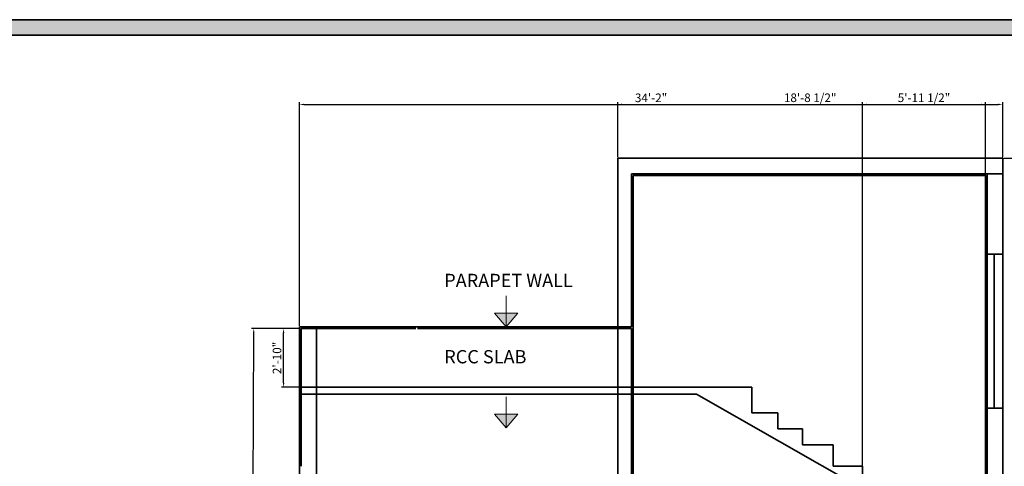
# Model space of a CAD drawing. Units: inches. Extents: x 1804 to 3296, y 909 to 2477.
# Tile 30 of 31: x 2434 to 3008, y 2216 to 2477. Entities that reach past the tile are written whole.
import ezdxf

# ---------------------------------------------------------------- set-up
doc = ezdxf.new("R2010")
doc.units = ezdxf.units.IN
for name, color, linetype, lineweight in [('A-ANNO-DIMS', 2, 'Continuous', 18), ('A-ANNO-SYMB', 7, 'Continuous', 18), ('A-ANNO-TTLB', 156, 'Continuous', 35), ('A-WALL-PATT', 10, 'Continuous', 13), ('SEC', 160, 'Continuous', 35), ('TEXT', 190, 'Continuous', 18)]:
    doc.layers.add(name, color=color, linetype=linetype, lineweight=lineweight)
doc.styles.get("Standard").update_dxf_attribs({"font": 'arial.ttf'})
doc.dimstyles.new('ISO-25', dxfattribs={"dimtxt": 5, "dimasz": 2.5, "dimexe": 1.25, "dimexo": 0.625, "dimtad": 1, "dimdec": 0, "dimlunit": 4, "dimtxsty": 'Standard', "dimcen": 2.5, "dimadec": 0, "dimazin": 0, "dimtfac": 1, "dimtdec": 0, "dimtmove": 0, "dimatfit": 3, "dimfxl": 1, "dimarcsym": 0})

# ---------------------------------------------------------------- blocks, each defined once
blk = doc.blocks.new('*D33')
at = {"layer": 'A-ANNO-DIMS', "color": 0, "lineweight": -2, "transparency": 16777216}
for p, q in [((3007.45, 2395.8), (3058.21, 2395.8)), ((3056.96, 1983.77), (3056.96, 2393.3)), ((3007.45, 1981.27), (3058.21, 1981.27))]:
    blk.add_line(p, q, dxfattribs=at)
at = {"layer": 'A-ANNO-DIMS', "color": 0, "lineweight": 100, "transparency": 16777216}
for points in [[(3056.55, 2393.3), (3057.38, 2393.3), (3056.96, 2395.8)], [(3056.55, 1983.77), (3057.38, 1983.77), (3056.96, 1981.27)]]:
    blk.add_solid(points, dxfattribs=at)
at = {"layer": 'Defpoints', "color": 0, "lineweight": 100, "transparency": 16777216}
for p in [(3006.82, 2395.8), (3056.96, 2395.8), (3006.82, 1981.27)]:
    blk.add_point(p, dxfattribs=at)
at = {"layer": 'A-ANNO-DIMS', "color": 0, "transparency": 16777216, "insert": (3053.79, 2188.53), "char_height": 5, "attachment_point": 5, "rotation": 90}
blk.add_mtext('34\'-7"', dxfattribs=at)
blk = doc.blocks.new('*D34')
at = {"layer": 'A-ANNO-DIMS', "color": 0, "lineweight": -2, "transparency": 16777216}
for p, q in [((2597.24, 2296.57), (2568.96, 2296.69)), ((2569.22, 2055.41), (2570.2, 2294.18)), ((2596.24, 2052.8), (2567.96, 2052.92))]:
    blk.add_line(p, q, dxfattribs=at)
at = {"layer": 'A-ANNO-DIMS', "color": 0, "lineweight": 100, "transparency": 16777216}
for points in [[(2569.78, 2294.19), (2570.61, 2294.18), (2570.21, 2296.68)], [(2568.8, 2055.41), (2569.64, 2055.41), (2569.21, 2052.91)]]:
    blk.add_solid(points, dxfattribs=at)
at = {"layer": 'Defpoints', "color": 0, "lineweight": 100, "transparency": 16777216}
for p in [(2570.21, 2296.68), (2597.87, 2296.57), (2596.87, 2052.8)]:
    blk.add_point(p, dxfattribs=at)
at = {"layer": 'A-ANNO-DIMS', "color": 0, "transparency": 16777216, "insert": (2566.53, 2174.81), "char_height": 5, "attachment_point": 5, "rotation": 89.76496}
blk.add_mtext('20\'-4"', dxfattribs=at)
blk = doc.blocks.new('*D35')
at = {"layer": 'A-ANNO-DIMS', "color": 0, "lineweight": -2, "transparency": 16777216}
for p, q in [((2597.24, 2296.57), (2586.36, 2296.57)), ((2587.61, 2264.89), (2587.61, 2294.07)), ((2597.24, 2262.39), (2586.36, 2262.39))]:
    blk.add_line(p, q, dxfattribs=at)
at = {"layer": 'A-ANNO-DIMS', "color": 0, "lineweight": 100, "transparency": 16777216}
for points in [[(2587.19, 2294.07), (2588.03, 2294.07), (2587.61, 2296.57)], [(2587.19, 2264.89), (2588.03, 2264.89), (2587.61, 2262.39)]]:
    blk.add_solid(points, dxfattribs=at)
at = {"layer": 'Defpoints', "color": 0, "lineweight": 100, "transparency": 16777216}
for p in [(2587.61, 2296.57), (2597.87, 2296.57), (2597.87, 2262.39)]:
    blk.add_point(p, dxfattribs=at)
at = {"layer": 'A-ANNO-DIMS', "color": 0, "transparency": 16777216, "insert": (2584.43, 2279.48), "char_height": 5, "attachment_point": 5, "rotation": 90}
blk.add_mtext('2\'-10"', dxfattribs=at)
blk = doc.blocks.new('SECTION-NOTE-ARROW')
h = blk.add_hatch(color=256)
h.dxf.hatch_style = 1
h.paths.add_polyline_path([(6.75, 8.05), (0, 8.05), (6.75, 0)])
h.paths.add_polyline_path([(13.51, 8.05), (6.75, 8.05), (6.75, 0)])
for p, q in [((6.75, 18.17), (6.75, 0)), ((6.75, 0), (0, 8.05)), ((0, 8.05), (13.51, 8.05)), ((6.75, 0), (13.51, 8.05))]:
    blk.add_line(p, q)
blk = doc.blocks.new('*D88')
at = {"layer": 'A-ANNO-DIMS', "color": 0, "lineweight": -2, "transparency": 16777216}
for p, q in [((2596.87, 2298.2), (2596.87, 2428.45)), ((3006.82, 2396.42), (3006.82, 2428.45)), ((2599.37, 2427.2), (3004.32, 2427.2))]:
    blk.add_line(p, q, dxfattribs=at)
at = {"layer": 'A-ANNO-DIMS', "color": 0, "lineweight": 100, "transparency": 16777216}
for points in [[(2599.37, 2427.61), (2599.37, 2426.78), (2596.87, 2427.2)], [(3004.32, 2427.61), (3004.32, 2426.78), (3006.82, 2427.2)]]:
    blk.add_solid(points, dxfattribs=at)
at = {"layer": 'Defpoints', "color": 0, "lineweight": 100, "transparency": 16777216}
for p in [(3006.82, 2427.2), (3006.82, 2395.8), (2596.87, 2297.57)]:
    blk.add_point(p, dxfattribs=at)
at = {"layer": 'A-ANNO-DIMS', "color": 0, "transparency": 16777216, "insert": (2801.84, 2430.38), "char_height": 5, "attachment_point": 5}
blk.add_mtext('34\'-2"', dxfattribs=at)
blk = doc.blocks.new('*D89')
at = {"layer": 'A-ANNO-DIMS', "color": 0, "lineweight": -2, "transparency": 16777216}
for p, q in [((2782.37, 2396.42), (2782.37, 2428.45)), ((3006.82, 2396.42), (3006.82, 2428.45)), ((2784.87, 2427.2), (3004.32, 2427.2))]:
    blk.add_line(p, q, dxfattribs=at)
at = {"layer": 'A-ANNO-DIMS', "color": 0, "lineweight": 100, "transparency": 16777216}
for points in [[(2784.87, 2427.61), (2784.87, 2426.78), (2782.37, 2427.2)], [(3004.32, 2427.61), (3004.32, 2426.78), (3006.82, 2427.2)]]:
    blk.add_solid(points, dxfattribs=at)
at = {"layer": 'Defpoints', "color": 0, "lineweight": 100, "transparency": 16777216}
for p in [(3006.82, 2427.2), (2782.37, 2395.8), (3006.82, 2395.8)]:
    blk.add_point(p, dxfattribs=at)
at = {"layer": 'A-ANNO-DIMS', "color": 0, "transparency": 16777216, "insert": (2894.59, 2430.41), "char_height": 5, "attachment_point": 5}
blk.add_mtext('18\'-8 1/2"', dxfattribs=at)
blk = doc.blocks.new('*D92')
at = {"layer": 'A-ANNO-DIMS', "color": 0, "lineweight": -2, "transparency": 16777216}
for p, q in [((2925.08, 2203.82), (2925.08, 2428.45)), ((2996.82, 2203.82), (2996.82, 2428.45)), ((2927.58, 2427.2), (2994.32, 2427.2))]:
    blk.add_line(p, q, dxfattribs=at)
at = {"layer": 'A-ANNO-DIMS', "color": 0, "lineweight": 100, "transparency": 16777216}
for points in [[(2927.58, 2427.61), (2927.58, 2426.78), (2925.08, 2427.2)], [(2994.32, 2427.61), (2994.32, 2426.78), (2996.82, 2427.2)]]:
    blk.add_solid(points, dxfattribs=at)
at = {"layer": 'Defpoints', "color": 0, "lineweight": 100, "transparency": 16777216}
for p in [(2996.82, 2427.2), (2925.08, 2203.2), (2996.82, 2203.2)]:
    blk.add_point(p, dxfattribs=at)
at = {"layer": 'A-ANNO-DIMS', "color": 0, "transparency": 16777216, "insert": (2960.95, 2430.41), "char_height": 5, "attachment_point": 5}
blk.add_mtext('5\'-11 1/2"', dxfattribs=at)

msp = doc.modelspace()

# ---------------------------------------------------------------- hatches: boundary and pattern name
at = {"layer": 'A-ANNO-TTLB'}
h = msp.add_hatch(color=256, dxfattribs=at)
h.dxf.hatch_style = 1
h.paths.add_polyline_path([(3294.53, 2476.54), (1803.79, 2476.54), (1805.43, 909.47), (3296.17, 909.47)])
h.paths.add_polyline_path([(1811, 914.33), (1812.79, 2467.54), (3285.53, 2467.54), (3283.74, 914.33)], flags=16)
h.paths.add_polyline_path([(1925.58, 1062.77), (1925.58, 1138.07), (1925.58, 1539.88), (1925.58, 1793.38), (1925.58, 1830.04), (2325.54, 1830.04), (2325.54, 1793.38), (2325.54, 1586.42), (2325.54, 1138.07), (2325.54, 1062.77)], flags=0)
h.paths.add_polyline_path([(1997.22, 1029.4), (2008.85, 1037.96), (2008.85, 1020.84)], flags=0)
h.paths.add_polyline_path([(1934.58, 1138.07), (1934.58, 1147.07), (2078.77, 1147.07), (2078.77, 1138.07), (2060.94, 1138.07)], flags=0)
h.paths.add_polyline_path([(1944.35, 1138.07), (1944.35, 1147.07), (2056.05, 1147.07), (2056.05, 1138.07)], flags=0)
h.paths.add_polyline_path([(2222.24, 1037.96), (2233.87, 1029.4), (2222.24, 1020.84)], flags=0)
h.paths.add_polyline_path([(2061.94, 1139.07), (2061.94, 1146.07), (2077.77, 1146.07), (2077.77, 1139.07)], flags=0)
h.paths.add_polyline_path([(2149.58, 1138.07), (2149.58, 1269.44), (2158.58, 1269.44), (2158.58, 1326.69), (2149.58, 1326.69), (2149.58, 1340.94), (2139.6, 1340.94), (2139.6, 1434.25), (2149.58, 1434.25), (2149.58, 1447.36), (2158.58, 1447.36), (2158.58, 1423.87), (2158.58, 1408.06), (2198.46, 1408.06), (2198.46, 1412.56), (2282.65, 1412.56), (2282.65, 1465.94), (2316.54, 1465.94), (2316.54, 1590.92), (2192.86, 1590.92), (2192.86, 1595.3), (2291.17, 1595.3), (2291.17, 1590.92), (2316.54, 1590.92), (2316.54, 1784.38), (2300.24, 1784.38), (2300.24, 1757.47), (2268, 1757.47), (2268, 1681.04), (2180.87, 1681.04), (2180.87, 1757.47), (2148.63, 1757.47), (2148.63, 1784.38), (2119.08, 1784.38), (2119.08, 1585.58), (2114.58, 1585.58), (2114.58, 1784.38), (2064.11, 1784.38), (2046.28, 1784.38), (2046.28, 1760.38), (1958.58, 1760.38), (1958.58, 1664.38), (1934.58, 1664.38), (1934.58, 1784.38), (1934.58, 1793.38), (2046.28, 1793.38), (2064.11, 1793.38), (2119.08, 1793.38), (2230.78, 1793.38), (2230.78, 1784.38), (2268, 1784.38), (2300.24, 1784.38), (2316.54, 1784.38), (2316.54, 1590.92), (2316.54, 1373.73), (2316.54, 1138.07)], flags=0)
h.paths.add_polyline_path([(2209.19, 1166.63), (2209.19, 1175.63), (2158.58, 1175.63), (2209.19, 1223.63), (2209.19, 1231.63), (2183.88, 1231.63), (2183.88, 1301.66), (2242.59, 1301.66), (2242.59, 1326.69), (2316.54, 1326.69), (2272.59, 1271.63), (2272.59, 1223.63), (2316.54, 1175.63), (2272.59, 1175.63), (2272.59, 1166.63)], flags=0)
h.paths.add_polyline_path([(1947.77, 1345.22), (1947.77, 1457.48), (1991.2, 1457.48), (1991.2, 1451.7), (1991.2, 1352.18), (1991.2, 1345.22)], flags=0)
h.paths.add_polyline_path([(2209.19, 1271.63), (2262.59, 1271.63), (2262.59, 1311.85), (2272.59, 1301.66), (2272.59, 1271.63), (2269.92, 1269.63), (2270.59, 1269.63), (2270.59, 1225.63), (2211.19, 1225.63), (2211.19, 1269.63), (2211.86, 1269.63)], flags=0)
h.paths.add_polyline_path([(2000.34, 1378.21), (2000.34, 1429.71), (2025.22, 1429.71), (2025.22, 1378.21)], flags=0)
h.paths.add_polyline_path([(2001.34, 1379.21), (2001.34, 1428.71), (2024.22, 1428.71), (2024.22, 1379.21)], flags=0)
h.paths.add_polyline_path([(2012.34, 1390.21), (2012.34, 1417.71), (2013.22, 1417.71), (2013.22, 1390.21)], flags=0)
h.paths.add_polyline_path([(2237.56, 1331.19), (2237.56, 1340.18), (2238.62, 1340.18), (2238.62, 1386.84), (2241.04, 1386.84), (2242.06, 1386.84), (2242.06, 1408.06), (2316.54, 1331.19)], flags=0)
h.paths.add_polyline_path([(1953.73, 1464.35), (1953.73, 1498.59), (1981.74, 1498.59), (1981.74, 1464.35)], flags=0)
h.paths.add_polyline_path([(1987.63, 1462.08), (1987.63, 1500.95), (2104.07, 1500.95), (2104.07, 1462.08), (2099.27, 1462.08), (1993.6, 1462.08)], flags=0)
h.paths.add_polyline_path([(1956.06, 1481.47, -1), (1979.41, 1481.47, -1)], flags=0)
edge = h.paths.add_edge_path(flags=0)
edge.add_ellipse((2299.53, 1438.37), major_axis=(0.31, 21.36), ratio=0.670333, start_angle=0, end_angle=360)
h.paths.add_polyline_path([(2297.39, 1438.37, -1), (2301.67, 1438.37, -1)], flags=0)
h.paths.add_polyline_path([(2591.54, 1163.23), (2591.54, 1179.38), (2591.54, 1379.68), (2591.54, 1395.84), (2734.5, 1395.84), (2734.5, 1379.68), (2734.5, 1179.38), (2734.5, 1163.23)], flags=0)
h.paths.add_polyline_path([(2592.54, 1164.23), (2592.54, 1166.23), (2733.5, 1166.23), (2733.5, 1164.23)], flags=0)
h.paths.add_polyline_path([(2592.54, 1180.38), (2592.54, 1378.68), (2733.5, 1378.68), (2733.5, 1180.38)], flags=0)
h.paths.add_polyline_path([(2593.54, 1181.38), (2593.54, 1377.68), (2732.5, 1377.68), (2732.5, 1181.38)], flags=0)
h.paths.add_polyline_path([(2594.54, 1182.38), (2594.54, 1376.68), (2731.5, 1376.68), (2731.5, 1182.38)], flags=0)
h.paths.add_polyline_path([(1936.95, 1697.46), (1936.95, 1736.46), (1955.41, 1736.46), (1955.41, 1697.46)], flags=0)
h.paths.add_polyline_path([(1938.48, 1718.36), (1938.48, 1734.92), (1953.65, 1734.92), (1953.65, 1718.36)], flags=0)
h.paths.add_polyline_path([(1944.75, 1726.64, -1), (1947.37, 1726.64, -1)], flags=0)
h.paths.add_polyline_path([(2592.54, 1394.84), (2733.5, 1394.84), (2733.5, 1392.84), (2592.54, 1392.84)], flags=0)
h.paths.add_polyline_path([(1976.61, 1762.5), (1976.61, 1781.44), (2012.79, 1781.44), (2012.79, 1762.5)], flags=0)
h.paths.add_polyline_path([(1979.57, 1771.97, -1), (1991.39, 1771.97, -1)], flags=0)
h.paths.add_polyline_path([(1995.36, 1771.97, -1), (2007.18, 1771.97, -1)], flags=0)
h.paths.add_polyline_path([(2251.51, 1744.53), (2268, 1730.05), (2251.51, 1730.05)], flags=0)
h.paths.add_polyline_path([(2047.28, 1785.38), (2047.28, 1792.38), (2063.11, 1792.38), (2063.11, 1785.38)], flags=0)
h.paths.add_polyline_path([(2155.08, 1770.92, -1), (2174.42, 1770.92, -1)], flags=0)
h.paths.add_polyline_path([(2188.59, 1758.27), (2188.59, 1772.81), (2222.3, 1772.81), (2222.3, 1758.27)], flags=0)
h.paths.add_polyline_path([(2223.97, 1758.27), (2223.97, 1772.81), (2257.68, 1772.81), (2257.68, 1758.27)], flags=0)
h.paths.add_polyline_path([(2274.45, 1770.92, -1), (2293.8, 1770.92, -1)], flags=0)
h.paths.add_polyline_path([(2591.54, 1582.09), (2591.54, 1782.39), (2734.5, 1782.39), (2734.5, 1582.09)], flags=0)
h.paths.add_polyline_path([(2592.54, 1583.09), (2592.54, 1781.39), (2733.5, 1781.39), (2733.5, 1583.09)], flags=0)
h.paths.add_polyline_path([(2593.54, 1584.09), (2593.54, 1780.39), (2732.5, 1780.39), (2732.5, 1584.09)], flags=0)
h.paths.add_polyline_path([(2594.54, 1585.09), (2594.54, 1779.39), (2731.5, 1779.39), (2731.5, 1585.09)], flags=0)
h.paths.add_polyline_path([(1922.17, 1978.79), (1922.17, 2295.08), (1922.17, 2296.08), (2115.67, 2296.08), (2115.67, 2384.31), (2115.67, 2385.31), (2322.12, 2385.31), (2323.12, 2385.31), (2323.12, 1979.79), (2323.12, 1978.79), (1923.17, 1978.79)], flags=0)
h.paths.add_polyline_path([(1922.17, 1978.79), (1922.17, 2051.31), (1922.17, 2214.86), (1922.17, 2296.08), (2115.67, 2296.08), (2115.67, 2385.31), (2323.12, 2385.31), (2323.12, 2280.42), (2323.12, 1978.79), (2115.67, 1978.79)], flags=0)
h.paths.add_polyline_path([(1923.17, 1979.79), (1923.17, 2050.31), (2115.67, 2050.31), (2115.67, 2051.31), (1923.17, 2051.31), (1923.17, 2213.86), (1923.17, 2214.86), (1923.17, 2295.08), (1990.02, 2295.08), (1990.02, 2214.86), (1991.02, 2214.86), (1991.02, 2295.08), (2115.67, 2295.08), (2115.67, 1979.79), (2116.67, 1979.79), (2116.67, 2304.18), (2116.67, 2384.31), (2322.12, 2384.31), (2322.12, 2280.42), (2322.12, 1979.79), (2115.67, 1979.79)], flags=0)
h.paths.add_polyline_path([(2972.46, 1192.5), (2972.46, 1196.92), (2995.47, 1196.92), (2995.47, 1255.47), (2995.09, 1255.47), (2987.42, 1249.39), (2980.08, 1255.47), (2978.05, 1255.47), (2978.05, 1257.24), (2995.47, 1257.24), (2995.47, 1261.58), (3015.37, 1261.58), (3015.37, 1333.28), (3015.37, 1414.4), (3032.82, 1414.4), (3032.82, 1333.28), (3032.82, 1261.58), (3052.66, 1261.58), (3052.66, 1255.47), (3079.86, 1255.47), (3078.72, 1254.57), (3081.47, 1252.29), (3078.56, 1249.99), (3075.81, 1252.26), (3072.57, 1249.69), (3070.36, 1251.52), (3067.67, 1249.39), (3060.34, 1255.47), (3052.66, 1255.47), (3052.66, 1196.92), (3054.58, 1196.92), (3074, 1196.92), (3074, 1192.5), (3052.66, 1192.5), (2995.47, 1192.5)], flags=0)
h.paths.add_polyline_path([(2490.75, 1979.27), (2490.75, 1980.27), (2596.87, 1980.27), (2596.87, 2051.8), (2596.87, 2052.8), (2596.87, 2216.35), (2596.87, 2297.57), (2717.32, 2297.57), (2710.57, 2305.62), (2724.07, 2305.62), (2717.32, 2297.57), (2782.37, 2297.57), (2782.37, 2395.8), (3006.82, 2395.8), (3006.82, 1981.27), (3093.73, 1981.27), (3093.73, 1980.27), (3047.51, 1980.27), (3046.37, 1979.37), (3049.11, 1977.1), (3046.2, 1974.79), (3043.46, 1977.07), (3040.21, 1974.49), (3038, 1976.32), (3035.32, 1974.2), (3027.98, 1980.27), (2871.83, 1980.27), (2871.83, 1981.27), (2791.37, 1981.27), (2791.37, 2050.8), (2597.87, 2050.8), (2597.87, 1980.27), (2597.87, 1979.27), (2546.27, 1979.27), (2545.12, 1978.37), (2547.87, 1976.1), (2544.96, 1973.79), (2542.22, 1976.07), (2538.97, 1973.49), (2536.76, 1975.32), (2534.07, 1973.2), (2526.74, 1979.27)], flags=0)
h.paths.add_polyline_path([(2597.87, 2051.8), (2606.87, 2051.8), (2606.87, 2258.39), (2597.87, 2258.39), (2597.87, 2296.57), (2606.87, 2296.57), (2606.87, 2262.39), (2782.37, 2262.39), (2782.37, 2296.57), (2790.37, 2296.57), (2790.37, 2262.39), (2791.37, 2262.39), (2791.37, 2305.67), (2791.37, 2385.8), (2996.82, 2385.8), (2996.82, 2339.85), (3006.82, 2339.85), (3006.82, 2250.12), (2997.82, 2250.12), (2997.82, 1981.27), (2996.82, 1981.27), (2872.83, 1981.27), (2872.83, 1991.8), (2871.83, 1991.8), (2871.83, 2050.8), (2790.37, 2050.8), (2597.87, 2050.8)], flags=0)
h.paths.add_polyline_path([(2179.93, 2153.92), (2179.93, 2353.97), (2259.98, 2353.97), (2259.98, 2153.92)], flags=0)
h.paths.add_polyline_path([(2180.93, 2154.92), (2180.93, 2352.97), (2258.98, 2352.97), (2258.98, 2154.92)], flags=0)
h.paths.add_polyline_path([(2960.87, 1608.49), (2960.87, 1753.62), (3070.9, 1753.62), (3070.9, 1608.49)], flags=0)
h.paths.add_polyline_path([(2961.87, 1609.49), (2961.87, 1752.62), (3069.9, 1752.62), (3069.9, 1609.49)], flags=0)
h.paths.add_polyline_path([(2962.87, 1610.49), (2962.87, 1751.62), (3068.9, 1751.62), (3068.9, 1610.49)], flags=0)
h.paths.add_polyline_path([(2963.87, 1611.49), (2963.87, 1750.62), (3067.9, 1750.62), (3067.9, 1611.49)], flags=0)
h.paths.add_polyline_path([(2782.37, 2051.8), (2782.37, 2216.32), (2791.37, 2216.32), (2791.37, 2051.8), (2872.83, 2051.8), (2872.83, 2068.56), (2884.67, 2068.56), (2884.67, 2085.33), (2896.51, 2085.33), (2896.51, 2102.09), (2908.36, 2102.09), (2908.36, 2118.85), (2920.2, 2118.85), (2920.2, 2135.62), (2932.05, 2135.62), (2932.05, 2145.3), (2925.08, 2145.3), (2925.08, 2203.2), (2996.82, 2203.2), (2996.82, 2145.3), (2953.82, 2145.3), (2872.83, 2051.8), (2790.37, 2051.8)], flags=0)
h.paths.add_polyline_path([(2717.32, 2238.65), (2710.57, 2246.7), (2724.07, 2246.7)], flags=0)
h.paths.add_polyline_path([(2003.09, 1122.79), (2017.16, 1122.79), (2017.16, 1138.74), (2003.09, 1138.74)], flags=8)
h.paths.add_polyline_path([(2174.76, 1792.72), (2188.83, 1792.72), (2188.83, 1808.66), (2174.76, 1808.66)], flags=8)
h.paths.add_polyline_path([(1987.95, 1792.51), (2002.02, 1792.51), (2002.02, 1808.45), (1987.95, 1808.45)], flags=8)
h.paths.add_polyline_path([(2148.79, 1289.26), (2160.46, 1289.26), (2160.46, 1305.2), (2148.79, 1305.2)], flags=8)
h.paths.add_polyline_path([(2115.36, 1133.57), (2127.04, 1133.57), (2127.04, 1149.51), (2115.36, 1149.51)], flags=8)
h.paths.add_polyline_path([(2237.58, 1421.48), (2249.25, 1421.48), (2249.25, 1437.43), (2237.58, 1437.43)], flags=8)
h.paths.add_polyline_path([(2134.99, 1584.32), (2146.66, 1584.32), (2146.66, 1600.26), (2134.99, 1600.26)], flags=8)
h.paths.add_polyline_path([(2101.95, 1557.31), (2113.62, 1557.31), (2113.62, 1573.25), (2101.95, 1573.25)], flags=8)
h.paths.add_polyline_path([(2937.85, 1156.77), (3120.41, 1156.77), (3120.41, 1185.72), (2937.85, 1185.72)], flags=8)
h.paths.add_polyline_path([(2980.71, 1786.71), (3050.06, 1786.71), (3050.06, 1802.66), (2980.71, 1802.66)], flags=8)
h.paths.add_polyline_path([(2869.28, 1661.96), (2938.62, 1661.96), (2938.62, 1690.8), (2869.28, 1690.8)], flags=8)
h.paths.add_polyline_path([(3092.27, 1674.86), (3161.62, 1674.86), (3161.62, 1690.8), (3092.27, 1690.8)], flags=8)
h.paths.add_polyline_path([(2980.71, 1674.86), (3050.06, 1674.86), (3050.06, 1690.8), (2980.71, 1690.8)], flags=8)
h.paths.add_polyline_path([(2649.07, 1678.23), (2674.53, 1678.23), (2674.53, 1714.76), (2649.07, 1714.76)], flags=8)
h.paths.add_polyline_path([(2530.84, 1981.63), (2549.13, 1981.63), (2549.13, 1997.57), (2530.84, 1997.57)], flags=8)
h.paths.add_polyline_path([(3031.29, 1981.77), (3049.58, 1981.77), (3049.58, 1997.71), (3031.29, 1997.71)], flags=8)
h.paths.add_polyline_path([(2715.38, 1911.9), (2851.54, 1911.9), (2851.54, 1940.85), (2715.38, 1940.85)], flags=8)
h.paths.add_polyline_path([(2015.23, 1927.36), (2205.42, 1927.36), (2205.42, 1956.3), (2015.23, 1956.3)], flags=8)
h.paths.add_polyline_path([(2671.84, 2057.84), (2702.75, 2057.84), (2702.75, 2073.79), (2671.84, 2073.79)], flags=8)
h.paths.add_polyline_path([(2678.5, 2316.52), (2765.26, 2316.52), (2765.26, 2332.46), (2678.5, 2332.46)], flags=8)
h.paths.add_polyline_path([(2678.48, 2271.96), (2736.41, 2271.96), (2736.41, 2287.9), (2678.48, 2287.9)], flags=8)
h.paths.add_polyline_path([(2019.2, 972.79), (2243.21, 972.79), (2243.21, 1001.74), (2019.2, 1001.74)], flags=8)
h.paths.add_polyline_path([(2097.06, 1021.56), (2132.16, 1021.56), (2132.16, 1037.51), (2097.06, 1037.51)], flags=8)
h.paths.add_polyline_path([(2182.47, 1360.48), (2207.35, 1360.48), (2207.35, 1376.42), (2182.47, 1376.42)], flags=8)
h.paths.add_polyline_path([(2261.12, 1361.77), (2295.01, 1361.77), (2295.01, 1377.71), (2261.12, 1377.71)], flags=8)
h.paths.add_polyline_path([(2245.75, 1511.51), (2278.44, 1511.51), (2278.44, 1527.46), (2245.75, 1527.46)], flags=8)
h.paths.add_polyline_path([(1991.16, 1296.29), (2060.51, 1296.29), (2060.51, 1312.23), (1991.16, 1312.23)], flags=8)
h.paths.add_polyline_path([(2187, 1651.35), (2246.71, 1651.35), (2246.71, 1667.29), (2187, 1667.29)], flags=8)
h.paths.add_polyline_path([(1976.49, 1684.81), (2068.63, 1684.81), (2068.63, 1700.76), (1976.49, 1700.76)], flags=8)
at = {"layer": 'A-WALL-PATT'}
h = msp.add_hatch(color=256, dxfattribs=at)
h.dxf.hatch_style = 1
h.paths.add_polyline_path([(2119.08, 1544.38), (1925.58, 1544.38), (1925.58, 1539.88), (2119.08, 1539.88)])
h.paths.add_polyline_path([(2119.08, 1545.58), (2114.58, 1545.58), (2114.58, 1544.38), (2119.08, 1544.38)])
h.paths.add_polyline_path([(1965.87, 1658.79), (1965.87, 1679.09), (1955.57, 1679.09), (1955.57, 1658.79)], flags=9)
h.paths.add_polyline_path([(2293.18, 1677.29), (2293.18, 1697.58), (2282.88, 1697.58), (2282.88, 1677.29)], flags=9)
h.paths.add_polyline_path([(2271.13, 1545.23), (2287.53, 1545.23), (2287.53, 1555.53), (2271.13, 1555.53)], flags=9)
h.paths.add_polyline_path([(2303.26, 1488.52), (2303.26, 1508.82), (2292.95, 1508.82), (2292.95, 1488.52)], flags=9)
h.paths.add_polyline_path([(2271.13, 1393.15), (2287.53, 1393.15), (2287.53, 1403.45), (2271.13, 1403.45)], flags=9)
h.paths.add_polyline_path([(2306.48, 1361.45), (2306.48, 1377.86), (2296.18, 1377.86), (2296.18, 1361.45)], flags=9)
h.paths.add_polyline_path([(2174.54, 1361.45), (2174.54, 1377.86), (2164.23, 1377.86), (2164.23, 1361.45)], flags=9)
h.paths.add_polyline_path([(1968.21, 1333.34), (1968.21, 1353.64), (1957.91, 1353.64), (1957.91, 1333.34)], flags=9)
h.paths.add_polyline_path([(2003.09, 1122.79), (2017.16, 1122.79), (2017.16, 1138.74), (2003.09, 1138.74)], flags=9)
h.paths.add_polyline_path([(2174.76, 1792.72), (2188.83, 1792.72), (2188.83, 1808.66), (2174.76, 1808.66)], flags=9)
h.paths.add_polyline_path([(1987.95, 1792.51), (2002.02, 1792.51), (2002.02, 1808.45), (1987.95, 1808.45)], flags=9)
h.paths.add_polyline_path([(2148.79, 1289.26), (2160.46, 1289.26), (2160.46, 1305.2), (2148.79, 1305.2)], flags=9)
h.paths.add_polyline_path([(2115.36, 1133.57), (2127.04, 1133.57), (2127.04, 1149.51), (2115.36, 1149.51)], flags=9)
h.paths.add_polyline_path([(2237.58, 1421.48), (2249.25, 1421.48), (2249.25, 1437.43), (2237.58, 1437.43)], flags=9)
h.paths.add_polyline_path([(2134.99, 1584.32), (2146.66, 1584.32), (2146.66, 1600.26), (2134.99, 1600.26)], flags=9)
h.paths.add_polyline_path([(2101.95, 1557.31), (2113.62, 1557.31), (2113.62, 1573.25), (2101.95, 1573.25)], flags=9)
h.paths.add_polyline_path([(2937.85, 1156.77), (3120.41, 1156.77), (3120.41, 1185.72), (2937.85, 1185.72)], flags=9)
h.paths.add_polyline_path([(2980.71, 1786.71), (3050.06, 1786.71), (3050.06, 1802.66), (2980.71, 1802.66)], flags=9)
h.paths.add_polyline_path([(2869.28, 1661.96), (2938.62, 1661.96), (2938.62, 1690.8), (2869.28, 1690.8)], flags=9)
h.paths.add_polyline_path([(3092.27, 1674.86), (3161.62, 1674.86), (3161.62, 1690.8), (3092.27, 1690.8)], flags=9)
h.paths.add_polyline_path([(2980.71, 1674.86), (3050.06, 1674.86), (3050.06, 1690.8), (2980.71, 1690.8)], flags=9)
h.paths.add_polyline_path([(2649.07, 1678.23), (2674.53, 1678.23), (2674.53, 1714.76), (2649.07, 1714.76)], flags=9)
h.paths.add_polyline_path([(2530.84, 1981.63), (2549.13, 1981.63), (2549.13, 1997.57), (2530.84, 1997.57)], flags=9)
h.paths.add_polyline_path([(3031.29, 1981.77), (3049.58, 1981.77), (3049.58, 1997.71), (3031.29, 1997.71)], flags=9)
h.paths.add_polyline_path([(2715.38, 1911.9), (2851.54, 1911.9), (2851.54, 1940.85), (2715.38, 1940.85)], flags=9)
h.paths.add_polyline_path([(2015.23, 1927.36), (2205.42, 1927.36), (2205.42, 1956.3), (2015.23, 1956.3)], flags=9)
h.paths.add_polyline_path([(2671.84, 2057.84), (2702.75, 2057.84), (2702.75, 2073.79), (2671.84, 2073.79)], flags=9)
h.paths.add_polyline_path([(2678.5, 2316.52), (2765.26, 2316.52), (2765.26, 2332.46), (2678.5, 2332.46)], flags=9)
h.paths.add_polyline_path([(2678.48, 2271.96), (2736.41, 2271.96), (2736.41, 2287.9), (2678.48, 2287.9)], flags=9)
h.paths.add_polyline_path([(2019.2, 972.79), (2243.21, 972.79), (2243.21, 1001.74), (2019.2, 1001.74)], flags=9)
h.paths.add_polyline_path([(2097.06, 1021.56), (2132.16, 1021.56), (2132.16, 1037.51), (2097.06, 1037.51)], flags=9)
h.paths.add_polyline_path([(2182.47, 1360.48), (2207.35, 1360.48), (2207.35, 1376.42), (2182.47, 1376.42)], flags=9)
h.paths.add_polyline_path([(2261.12, 1361.77), (2295.01, 1361.77), (2295.01, 1377.71), (2261.12, 1377.71)], flags=9)
h.paths.add_polyline_path([(2245.75, 1511.51), (2278.44, 1511.51), (2278.44, 1527.46), (2245.75, 1527.46)], flags=9)
h.paths.add_polyline_path([(1991.16, 1296.29), (2060.51, 1296.29), (2060.51, 1312.23), (1991.16, 1312.23)], flags=9)
h.paths.add_polyline_path([(2187, 1651.35), (2246.71, 1651.35), (2246.71, 1667.29), (2187, 1667.29)], flags=9)
h.paths.add_polyline_path([(1976.49, 1684.81), (2068.63, 1684.81), (2068.63, 1700.76), (1976.49, 1700.76)], flags=9)
h = msp.add_hatch(color=256, dxfattribs=at)
h.dxf.hatch_style = 1
h.paths.add_polyline_path([(2149.58, 1147.07), (2141.21, 1147.07), (2141.21, 1144.07), (2141.21, 1138.07), (2149.58, 1138.07)])
h.paths.add_polyline_path([(2101.21, 1144.07, -0.01877), (2101.32, 1147.07), (2078.77, 1147.07), (2078.77, 1138.07), (2101.21, 1138.07)])
h.paths.add_polyline_path([(2060.94, 1147.07), (2056.05, 1147.07), (2056.05, 1138.07), (2060.94, 1138.07)])
h.paths.add_polyline_path([(1944.35, 1147.07), (1934.58, 1147.07), (1934.58, 1138.07), (1944.35, 1138.07)])
h.paths.add_polyline_path([(2158.58, 1269.44), (2149.58, 1269.44), (2149.58, 1138.07), (2158.58, 1138.07)])
h.paths.add_polyline_path([(2003.09, 1122.79), (2017.16, 1122.79), (2017.16, 1138.74), (2003.09, 1138.74)], flags=9)
h.paths.add_polyline_path([(2174.76, 1792.72), (2188.83, 1792.72), (2188.83, 1808.66), (2174.76, 1808.66)], flags=9)
h.paths.add_polyline_path([(1987.95, 1792.51), (2002.02, 1792.51), (2002.02, 1808.45), (1987.95, 1808.45)], flags=9)
h.paths.add_polyline_path([(2148.79, 1289.26), (2160.46, 1289.26), (2160.46, 1305.2), (2148.79, 1305.2)], flags=9)
h.paths.add_polyline_path([(2115.36, 1133.57), (2127.04, 1133.57), (2127.04, 1149.51), (2115.36, 1149.51)], flags=9)
h.paths.add_polyline_path([(2237.58, 1421.48), (2249.25, 1421.48), (2249.25, 1437.43), (2237.58, 1437.43)], flags=9)
h.paths.add_polyline_path([(2134.99, 1584.32), (2146.66, 1584.32), (2146.66, 1600.26), (2134.99, 1600.26)], flags=9)
h.paths.add_polyline_path([(2101.95, 1557.31), (2113.62, 1557.31), (2113.62, 1573.25), (2101.95, 1573.25)], flags=9)
h.paths.add_polyline_path([(2937.85, 1156.77), (3120.41, 1156.77), (3120.41, 1185.72), (2937.85, 1185.72)], flags=9)
h.paths.add_polyline_path([(2980.71, 1786.71), (3050.06, 1786.71), (3050.06, 1802.66), (2980.71, 1802.66)], flags=9)
h.paths.add_polyline_path([(2869.28, 1661.96), (2938.62, 1661.96), (2938.62, 1690.8), (2869.28, 1690.8)], flags=9)
h.paths.add_polyline_path([(3092.27, 1674.86), (3161.62, 1674.86), (3161.62, 1690.8), (3092.27, 1690.8)], flags=9)
h.paths.add_polyline_path([(2980.71, 1674.86), (3050.06, 1674.86), (3050.06, 1690.8), (2980.71, 1690.8)], flags=9)
h.paths.add_polyline_path([(2649.07, 1678.23), (2674.53, 1678.23), (2674.53, 1714.76), (2649.07, 1714.76)], flags=9)
h.paths.add_polyline_path([(2530.84, 1981.63), (2549.13, 1981.63), (2549.13, 1997.57), (2530.84, 1997.57)], flags=9)
h.paths.add_polyline_path([(3031.29, 1981.77), (3049.58, 1981.77), (3049.58, 1997.71), (3031.29, 1997.71)], flags=9)
h.paths.add_polyline_path([(2715.38, 1911.9), (2851.54, 1911.9), (2851.54, 1940.85), (2715.38, 1940.85)], flags=9)
h.paths.add_polyline_path([(2015.23, 1927.36), (2205.42, 1927.36), (2205.42, 1956.3), (2015.23, 1956.3)], flags=9)
h.paths.add_polyline_path([(2671.84, 2057.84), (2702.75, 2057.84), (2702.75, 2073.79), (2671.84, 2073.79)], flags=9)
h.paths.add_polyline_path([(2678.5, 2316.52), (2765.26, 2316.52), (2765.26, 2332.46), (2678.5, 2332.46)], flags=9)
h.paths.add_polyline_path([(2678.48, 2271.96), (2736.41, 2271.96), (2736.41, 2287.9), (2678.48, 2287.9)], flags=9)
h.paths.add_polyline_path([(2019.2, 972.79), (2243.21, 972.79), (2243.21, 1001.74), (2019.2, 1001.74)], flags=9)
h.paths.add_polyline_path([(2097.06, 1021.56), (2132.16, 1021.56), (2132.16, 1037.51), (2097.06, 1037.51)], flags=9)
h.paths.add_polyline_path([(2182.47, 1360.48), (2207.35, 1360.48), (2207.35, 1376.42), (2182.47, 1376.42)], flags=9)
h.paths.add_polyline_path([(2261.12, 1361.77), (2295.01, 1361.77), (2295.01, 1377.71), (2261.12, 1377.71)], flags=9)
h.paths.add_polyline_path([(2245.75, 1511.51), (2278.44, 1511.51), (2278.44, 1527.46), (2245.75, 1527.46)], flags=9)
h.paths.add_polyline_path([(1991.16, 1296.29), (2060.51, 1296.29), (2060.51, 1312.23), (1991.16, 1312.23)], flags=9)
h.paths.add_polyline_path([(2187, 1651.35), (2246.71, 1651.35), (2246.71, 1667.29), (2187, 1667.29)], flags=9)
h.paths.add_polyline_path([(1976.49, 1684.81), (2068.63, 1684.81), (2068.63, 1700.76), (1976.49, 1700.76)], flags=9)
h = msp.add_hatch(color=256, dxfattribs=at)
h.dxf.hatch_style = 1
h.paths.add_polyline_path([(2158.58, 1275.49), (2155.29, 1275.49), (2149.58, 1275.49), (2149.58, 1269.44), (2158.58, 1269.44)])
h.paths.add_polyline_path([(2158.58, 1326.69), (2149.58, 1326.69), (2149.58, 1319.33), (2155.29, 1319.33), (2158.58, 1319.33)])
h.paths.add_polyline_path([(2158.58, 1402.2), (2158.58, 1423.87), (2158.58, 1447.36), (2149.58, 1447.36), (2149.58, 1423.87), (2149.58, 1340.94), (2149.58, 1326.69), (2158.58, 1326.69), (2158.58, 1354.23)])
h.paths.add_polyline_path([(1965.87, 1658.79), (1965.87, 1679.09), (1955.57, 1679.09), (1955.57, 1658.79)], flags=9)
h.paths.add_polyline_path([(2293.18, 1677.29), (2293.18, 1697.58), (2282.88, 1697.58), (2282.88, 1677.29)], flags=9)
h.paths.add_polyline_path([(2271.13, 1545.23), (2287.53, 1545.23), (2287.53, 1555.53), (2271.13, 1555.53)], flags=9)
h.paths.add_polyline_path([(2303.26, 1488.52), (2303.26, 1508.82), (2292.95, 1508.82), (2292.95, 1488.52)], flags=9)
h.paths.add_polyline_path([(2271.13, 1393.15), (2287.53, 1393.15), (2287.53, 1403.45), (2271.13, 1403.45)], flags=9)
h.paths.add_polyline_path([(2306.48, 1361.45), (2306.48, 1377.86), (2296.18, 1377.86), (2296.18, 1361.45)], flags=9)
h.paths.add_polyline_path([(2189.9, 1340.62), (2206.31, 1340.62), (2206.31, 1350.92), (2189.9, 1350.92)], flags=9)
h.paths.add_polyline_path([(2174.54, 1361.45), (2174.54, 1377.86), (2164.23, 1377.86), (2164.23, 1361.45)], flags=9)
h.paths.add_polyline_path([(2304.24, 1240.8), (2304.24, 1261.09), (2293.94, 1261.09), (2293.94, 1240.8)], flags=9)
h.paths.add_polyline_path([(2227.19, 1188.73), (2247.49, 1188.73), (2247.49, 1199.03), (2227.19, 1199.03)], flags=9)
h.paths.add_polyline_path([(2181.93, 1144.21), (2181.93, 1160.62), (2171.63, 1160.62), (2171.63, 1144.21)], flags=9)
h.paths.add_polyline_path([(1968.21, 1333.34), (1968.21, 1353.64), (1957.91, 1353.64), (1957.91, 1333.34)], flags=9)
h.paths.add_polyline_path([(2029.78, 1203.53), (2053.95, 1203.53), (2053.95, 1213.83), (2029.78, 1213.83)], flags=9)
h.paths.add_polyline_path([(2576.51, 1671.88), (2576.51, 1692.17), (2566.21, 1692.17), (2566.21, 1671.88)], flags=9)
h.paths.add_polyline_path([(2566.99, 1269.67), (2566.99, 1289.96), (2556.68, 1289.96), (2556.68, 1269.67)], flags=9)
h.paths.add_polyline_path([(2581.85, 1269.17), (2581.85, 1289.46), (2571.54, 1289.46), (2571.54, 1269.17)], flags=9)
h.paths.add_polyline_path([(2650.71, 1409.75), (2674.89, 1409.75), (2674.89, 1420.05), (2650.71, 1420.05)], flags=9)
h.paths.add_polyline_path([(2003.09, 1122.79), (2017.16, 1122.79), (2017.16, 1138.74), (2003.09, 1138.74)], flags=9)
h.paths.add_polyline_path([(2174.76, 1792.72), (2188.83, 1792.72), (2188.83, 1808.66), (2174.76, 1808.66)], flags=9)
h.paths.add_polyline_path([(1987.95, 1792.51), (2002.02, 1792.51), (2002.02, 1808.45), (1987.95, 1808.45)], flags=9)
h.paths.add_polyline_path([(2148.79, 1289.26), (2160.46, 1289.26), (2160.46, 1305.2), (2148.79, 1305.2)], flags=9)
h.paths.add_polyline_path([(2115.36, 1133.57), (2127.04, 1133.57), (2127.04, 1149.51), (2115.36, 1149.51)], flags=9)
h.paths.add_polyline_path([(2237.58, 1421.48), (2249.25, 1421.48), (2249.25, 1437.43), (2237.58, 1437.43)], flags=9)
h.paths.add_polyline_path([(2134.99, 1584.32), (2146.66, 1584.32), (2146.66, 1600.26), (2134.99, 1600.26)], flags=9)
h.paths.add_polyline_path([(2101.95, 1557.31), (2113.62, 1557.31), (2113.62, 1573.25), (2101.95, 1573.25)], flags=9)
h.paths.add_polyline_path([(2937.85, 1156.77), (3120.41, 1156.77), (3120.41, 1185.72), (2937.85, 1185.72)], flags=9)
h.paths.add_polyline_path([(2980.71, 1786.71), (3050.06, 1786.71), (3050.06, 1802.66), (2980.71, 1802.66)], flags=9)
h.paths.add_polyline_path([(2869.28, 1661.96), (2938.62, 1661.96), (2938.62, 1690.8), (2869.28, 1690.8)], flags=9)
h.paths.add_polyline_path([(3092.27, 1674.86), (3161.62, 1674.86), (3161.62, 1690.8), (3092.27, 1690.8)], flags=9)
h.paths.add_polyline_path([(2980.71, 1674.86), (3050.06, 1674.86), (3050.06, 1690.8), (2980.71, 1690.8)], flags=9)
h.paths.add_polyline_path([(2649.07, 1678.23), (2674.53, 1678.23), (2674.53, 1714.76), (2649.07, 1714.76)], flags=9)
h.paths.add_polyline_path([(2530.84, 1981.63), (2549.13, 1981.63), (2549.13, 1997.57), (2530.84, 1997.57)], flags=9)
h.paths.add_polyline_path([(3031.29, 1981.77), (3049.58, 1981.77), (3049.58, 1997.71), (3031.29, 1997.71)], flags=9)
h.paths.add_polyline_path([(2715.38, 1911.9), (2851.54, 1911.9), (2851.54, 1940.85), (2715.38, 1940.85)], flags=9)
h.paths.add_polyline_path([(2015.23, 1927.36), (2205.42, 1927.36), (2205.42, 1956.3), (2015.23, 1956.3)], flags=9)
h.paths.add_polyline_path([(2671.84, 2057.84), (2702.75, 2057.84), (2702.75, 2073.79), (2671.84, 2073.79)], flags=9)
h.paths.add_polyline_path([(2678.5, 2316.52), (2765.26, 2316.52), (2765.26, 2332.46), (2678.5, 2332.46)], flags=9)
h.paths.add_polyline_path([(2678.48, 2271.96), (2736.41, 2271.96), (2736.41, 2287.9), (2678.48, 2287.9)], flags=9)
h.paths.add_polyline_path([(2019.2, 972.79), (2243.21, 972.79), (2243.21, 1001.74), (2019.2, 1001.74)], flags=9)
h.paths.add_polyline_path([(2097.06, 1021.56), (2132.16, 1021.56), (2132.16, 1037.51), (2097.06, 1037.51)], flags=9)
h.paths.add_polyline_path([(2182.47, 1360.48), (2207.35, 1360.48), (2207.35, 1376.42), (2182.47, 1376.42)], flags=9)
h.paths.add_polyline_path([(2261.12, 1361.77), (2295.01, 1361.77), (2295.01, 1377.71), (2261.12, 1377.71)], flags=9)
h.paths.add_polyline_path([(2245.75, 1511.51), (2278.44, 1511.51), (2278.44, 1527.46), (2245.75, 1527.46)], flags=9)
h.paths.add_polyline_path([(1991.16, 1296.29), (2060.51, 1296.29), (2060.51, 1312.23), (1991.16, 1312.23)], flags=9)
h.paths.add_polyline_path([(2187, 1651.35), (2246.71, 1651.35), (2246.71, 1667.29), (2187, 1667.29)], flags=9)
h.paths.add_polyline_path([(1976.49, 1684.81), (2068.63, 1684.81), (2068.63, 1700.76), (1976.49, 1700.76)], flags=9)

# ---------------------------------------------------------------- linework, layer by layer
at = {"layer": 'A-ANNO-TTLB'}
for points in [[(1803.79, 2476.54), (3294.53, 2476.54), (3296.17, 909.47), (1805.43, 909.47)], [(1812.79, 2467.54), (3285.53, 2467.54), (3283.74, 914.33), (1811, 914.33)]]:
    msp.add_lwpolyline(points, close=True, dxfattribs=at)
at = {"layer": 'SEC'}
for p, q in [((2782.37, 2395.8), (3006.82, 2395.8)), ((2782.37, 2297.57), (2782.37, 2395.8)), ((3006.82, 1981.27), (3006.82, 2395.8)), ((2790.37, 2297.57), (2790.37, 2386.8)), ((2790.37, 2386.8), (2997.82, 2386.8)), ((2791.37, 2297.57), (2791.37, 2385.8)), ((2791.37, 2385.8), (2996.82, 2385.8)), ((2996.82, 2385.8), (2996.82, 2281.91)), ((2997.82, 2386.8), (2997.82, 2281.91)), ((3006.82, 2386.8), (2997.82, 2386.8)), ((3006.82, 2385.8), (3006.82, 2386.8)), ((3001.82, 2250.12), (3001.82, 2339.85)), ((2782.37, 2051.8), (2782.37, 2305.67)), ((2790.37, 2297.57), (2790.37, 2305.67)), ((2791.37, 2051.8), (2791.37, 2305.67)), ((2596.87, 2216.35), (2596.87, 2297.57)), ((2596.87, 2297.57), (2790.37, 2297.57)), ((2597.87, 2216.35), (2597.87, 2296.57)), ((2597.87, 2296.57), (2664.71, 2296.57)), ((2606.87, 2051.8), (2606.87, 2296.57)), ((2665.71, 2296.57), (2790.37, 2296.57)), ((2790.37, 2051.8), (2790.37, 2296.57)), ((2996.82, 1981.27), (2996.82, 2281.91)), ((2997.82, 1981.27), (2997.82, 2281.91)), ((2791.37, 2262.39), (2597.87, 2262.39)), ((2791.37, 2262.39), (2860.51, 2262.39)), ((2860.51, 2262.39), (2860.6, 2256.93)), ((2791.37, 2258.39), (2597.87, 2258.39)), ((2828.35, 2258.39), (2791.37, 2258.39)), ((2925.08, 2203.2), (2828.35, 2258.39)), ((2860.6, 2247.43), (2860.6, 2256.93)), ((2875.7, 2247.43), (2860.6, 2247.43)), ((2875.7, 2238.07), (2875.7, 2247.43)), ((2890.08, 2238.07), (2875.7, 2238.07)), ((2890.08, 2228.85), (2890.08, 2238.07)), ((2907.97, 2228.85), (2890.08, 2228.85)), ((2907.97, 2216.5), (2907.97, 2228.85)), ((2596.87, 2052.8), (2596.87, 2216.35)), ((2913.55, 2216.5), (2907.97, 2216.5)), ((2925.08, 2216.5), (2913.55, 2216.5)), ((2925.08, 2203.2), (2925.08, 2216.5))]:
    msp.add_line(p, q, dxfattribs=at)
msp.add_lwpolyline([(2996.82, 2250.12), (3006.82, 2250.12), (3006.82, 2339.85), (2996.82, 2339.85)], close=True, dxfattribs=at)

# ---------------------------------------------------------------- block references
at = {"layer": 'A-ANNO-SYMB'}
for p in [(2710.57, 2297.57), (2710.57, 2238.65)]:
    msp.add_blockref('SECTION-NOTE-ARROW', p, dxfattribs=at)

# ---------------------------------------------------------------- texts
at = {"layer": 'TEXT', "attachment_point": 1}
for s, insert, char_height in [('PARAPET WALL', (2681.27, 2328.48), 7.7373), ('RCC SLAB', (2681.27, 2284.05), 7.737)]:
    msp.add_mtext_dynamic_manual_height_columns(s, width=163.3261, gutter_width=38.69, heights=[0], dxfattribs=dict(at, insert=insert, char_height=char_height))

# ---------------------------------------------------------------- dimensions: what is measured, and where the dimension line sits
at = {"layer": 'A-ANNO-DIMS'}
for base, p1, p2, picture, middle in [((3006.8203, 2427.1958), (2596.8657, 2297.5705), (3006.8203, 2395.7958), '*D88', (2801.843, 2430.3754)), ((3006.8203, 2427.1958), (2782.3657, 2395.7958), (3006.8203, 2395.7958), '*D89', (2894.593, 2430.4061)), ((2996.82, 2427.2), (2925.08, 2203.2), (2996.82, 2203.2), '*D92', (2960.95, 2430.41))]:
    dim = msp.add_linear_dim(base=base, p1=p1, p2=p2, dimstyle='ISO-25', override={"dimdec": 1, "dimlfac": 1, "dimrnd": 0, "dimzin": 1, "dimdsep": 46, "dimlunit": 4, "dimfrac": 2}, dxfattribs=at)
    dim.commit()
    dim.dimension.update_dxf_attribs({"geometry": picture, "text_midpoint": middle})
for base, p1, p2, picture, middle in [((3056.96, 2395.8), (3006.82, 1981.27), (3006.82, 2395.8), '*D33', (3053.79, 2188.53)), ((2587.61, 2296.57), (2597.87, 2262.39), (2597.87, 2296.57), '*D35', (2584.43, 2279.48))]:
    dim = msp.add_linear_dim(base=base, p1=p1, p2=p2, angle=90, dimstyle='ISO-25', override={"dimclrd": 0, "dimclre": 0, "dimclrt": 0}, dxfattribs=at)
    dim.commit()
    dim.dimension.update_dxf_attribs({"geometry": picture, "text_midpoint": middle})
dim = msp.add_aligned_dim(p1=(2596.87, 2052.8), p2=(2597.87, 2296.57), distance=27.66, dimstyle='ISO-25', override={"dimclrd": 0, "dimclre": 0, "dimclrt": 0}, dxfattribs=at)
dim.commit()
dim.dimension.update_dxf_attribs({"geometry": '*D34', "text_midpoint": (2566.53, 2174.81)})

doc.saveas('drawing.dxf')
